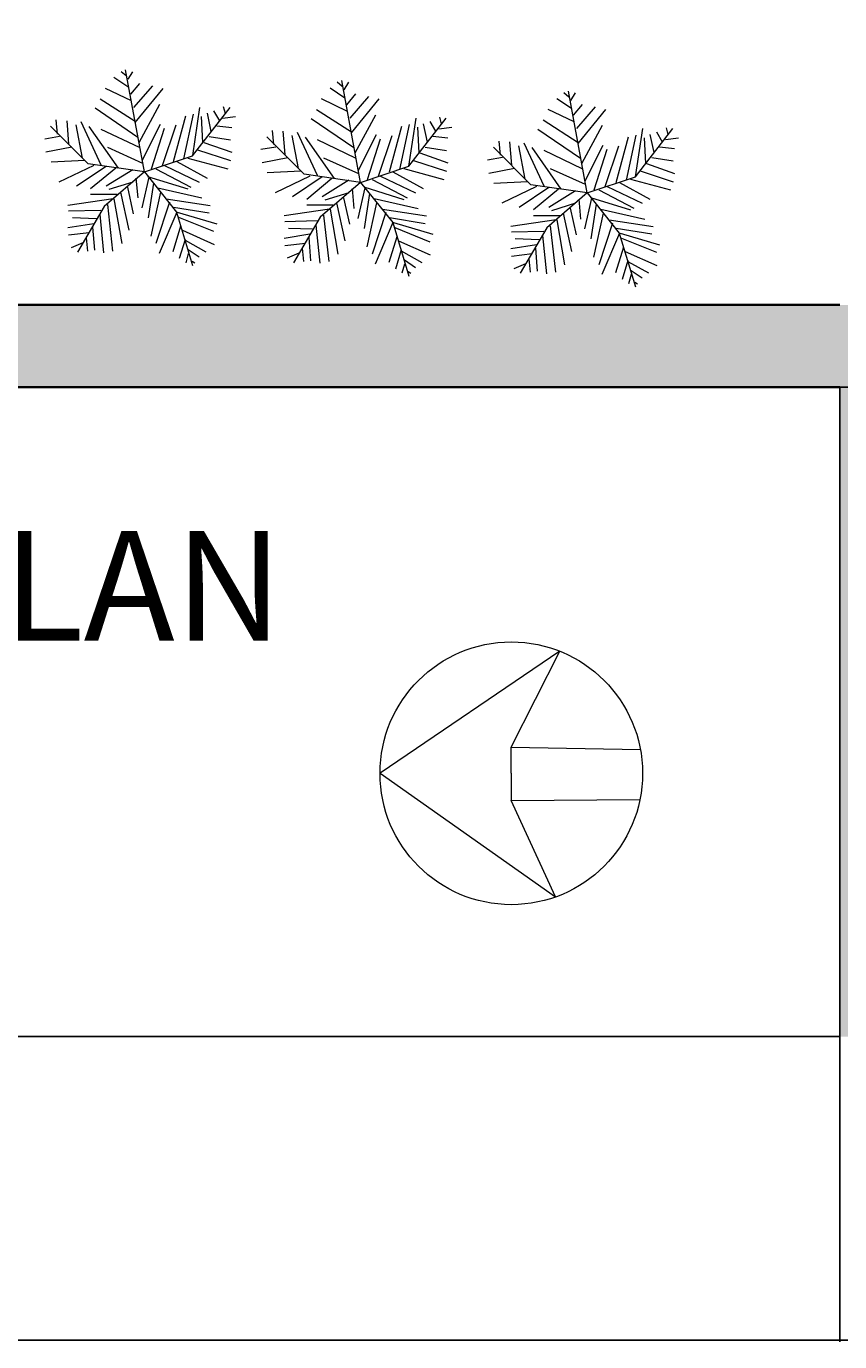
# Model space of a CAD drawing. Units: inches. Extents: x 2070 to 4408, y 1595 to 4269.
# Tile 4 of 20: x 2247 to 2336, y 1595 to 1739. Entities that reach past the tile are written whole.
import ezdxf

# ---------------------------------------------------------------- set-up
doc = ezdxf.new("R2010")
doc.units = ezdxf.units.IN
for name, color, linetype, lineweight in [('A-ANNO-DIMS', 2, 'Continuous', 18), ('A-ANNO-SYMB', 7, 'Continuous', 18), ('A-ANNO-TITL', 7, 'Continuous', 25), ('A-WALL', 7, 'Continuous', 35), ('L-PLNT', 3, 'Continuous', 13)]:
    doc.layers.add(name, color=color, linetype=linetype, lineweight=lineweight)
doc.layers.add('A-WALL-PATT', color=18, linetype='Continuous', lineweight=13, true_color=0x000000)
doc.styles.get("Standard").update_dxf_attribs({"font": 'arial.ttf'})
doc.dimstyles.get("Standard").update_dxf_attribs({"dimtxt": 0.18, "dimasz": 0.18, "dimexe": 0.18, "dimexo": 0.0625, "dimgap": 0.09, "dimtad": 0, "dimtih": 1, "dimtoh": 1, "dimdec": 4, "dimzin": 0, "dimdsep": 46, "dimtxsty": 'Standard', "dimcen": 0.09, "dimadec": 0, "dimazin": 0, "dimtfac": 1, "dimtdec": 4, "dimtofl": 0, "dimtmove": 0, "dimatfit": 3, "dimfxl": 1, "dimtolj": 1, "dimtzin": 0, "dimarcsym": 0})

# ---------------------------------------------------------------- blocks, each defined once
blk = doc.blocks.new('Trees - Imperial')
for p, q in [((-8.737, 47.138), (-17.069, 52.711)), ((-10.186, 53.64), (-13.084, 55.962)), ((0, 0), (-10.5, 57)), ((-9.099, 51.782), (-6.563, 55.962)), ((-7.288, 39.707), (-21.778, 46.673)), ((-7.65, 43.423), (-2.578, 49.46)), ((-5.839, 35.992), (4.667, 48.067)), ((-5.114, 27.632), (10.463, 46.673)), ((-5.114, 28.097), (-24.676, 40.636)), ((-2.941, 16.486), (8.652, 37.85)), ((-3.665, 19.273), (-27.574, 35.527)), ((16.259, 5.805), (23.142, 31.348)), ((22.055, 7.198), (27.489, 32.277)), ((27, 9), (48, 36)), ((27.127, 9.056), (31.112, 35.992)), ((31.836, 30.883), (32.561, 16.486)), ((35.096, 32.741), (37.27, 22.524)), ((38.719, 34.134), (41.979, 28.561)), ((43.791, 29.954), (51.036, 30.883)), ((44.153, 36.456), (45.239, 32.741)), ((-31.5, 4.5), (-52.5, 25.5)), ((-48.585, 21.131), (-49.309, 29.026)), ((-43.513, 28.561), (-42.427, 15.558)), ((-38.442, 26.239), (-34.819, 7.663)), ((-35.544, 28.097), (-24.314, 3.947)), ((-14.533, 2.09), (-30.834, 25.31)), ((-24.314, 23.917), (-2.941, 13.7)), ((-1.129, 6.734), (9.014, 26.704)), ((3.942, 1.625), (11.187, 24.381)), ((10.101, 3.483), (17.708, 26.239)), ((40.53, 25.775), (48.862, 24.846)), ((-47.498, 19.737), (-55.83, 18.344)), ((33.285, 16.486), (48.862, 10.913)), ((36.183, 19.737), (48.137, 17.88)), ((-40.615, 13.7), (-55.105, 10.913)), ((-20.691, 13.7), (-1.129, 4.876)), ((0, 0), (27, 9)), ((24.229, 7.663), (46.688, 1.625)), ((29.662, 12.307), (48.137, 6.269)), ((-33.37, 6.269), (-52.207, 5.34)), ((-28.299, 3.483), (-47.86, -5.805)), ((-21.416, 3.018), (-38.079, -8.128)), ((0, 0), (-31.5, 4.5)), ((-15.982, 2.09), (-30.11, -9.521)), ((0, 0), (-22.5, -19.5)), ((-6.563, 1.161), (-21.416, -8.128)), ((0, 0), (18, -22.5)), ((6.478, 1.625), (26.04, -8.592)), ((11.187, 3.483), (30.749, -5.805)), ((18.07, 5.805), (35.096, -3.483)), ((-6.563, -5.805), (-19.967, -9.985)), ((-4.752, -3.483), (-3.665, -14.629)), ((2.493, -3.019), (-1.491, -20.202)), ((1.769, -2.555), (24.229, -9.521)), ((5.029, -6.27), (2.131, -25.775)), ((-15.257, -12.772), (-30.11, -12.772)), ((-13.446, -11.378), (-8.737, -32.741)), ((-9.461, -8.592), (-6.201, -23.453)), ((9.014, -11.378), (3.58, -35.992)), ((7.565, -9.056), (32.198, -14.629)), ((-17.431, -15.094), (-42.789, -18.809)), ((-24.314, -21.596), (-42.427, -22.06)), ((-22.5, -19.5), (-37.5, -45)), ((-20.691, -18.345), (-17.793, -44.352)), ((-17.069, -15.094), (-12.721, -40.172)), ((14.085, -16.951), (6.478, -40.172)), ((12.274, -15.094), (36.907, -18.809)), ((16.259, -19.738), (36.183, -22.989)), ((-28.299, -29.026), (-42.789, -31.348)), ((-26.849, -26.24), (-40.253, -25.775)), ((-25.038, -23.918), (-22.865, -45.281)), ((18.07, -22.524), (8.289, -45.745)), ((18, -22.5), (27, -52.5)), ((18.433, -22.524), (40.53, -29.026)), ((19.157, -25.311), (38.719, -33.206)), ((-30.834, -34.135), (-42.427, -35.528)), ((-29.023, -30.884), (-27.936, -43.887)), ((20.244, -30.419), (15.897, -44.816)), ((21.331, -32.741), (39.081, -40.636)), ((-34.457, -39.708), (-40.978, -42.494)), ((-32.646, -36.921), (-31.921, -44.352)), ((22.78, -37.85), (19.519, -48.532)), ((22.78, -38.314), (34.372, -44.816)), ((24.591, -43.423), (30.749, -47.603)), ((24.591, -45.745), (23.142, -50.854)), ((26.764, -49.925), (28.213, -50.854))]:
    blk.add_line(p, q)
blk = doc.blocks.new('*D24')
at = {"layer": 'A-ANNO-DIMS', "color": 0, "lineweight": -2, "transparency": 16777216}
for p, q in [((2103.13, 2291.4), (2069.84, 2291.4)), ((2070.02, 2291.22), (2070.02, 1960.08)), ((2070.02, 1628.58), (2070.02, 1959.72)), ((2336.13, 1628.4), (2069.84, 1628.4))]:
    blk.add_line(p, q, dxfattribs=at)
at = {"layer": 'A-ANNO-DIMS', "color": 0, "transparency": 16777216}
for points in [[(2069.99, 2291.22), (2070.05, 2291.22), (2070.02, 2291.4)], [(2069.99, 1628.58), (2070.05, 1628.58), (2070.02, 1628.4)]]:
    blk.add_solid(points, dxfattribs=at)
at = {"layer": 'Defpoints', "color": 0, "transparency": 16777216}
for p in [(2070.02, 2291.4), (2103.2, 2291.4), (2336.2, 1628.4)]:
    blk.add_point(p, dxfattribs=at)
at = {"layer": 'A-ANNO-DIMS', "color": 0, "transparency": 16777216, "insert": (2070.02, 1959.9), "char_height": 0.18, "attachment_point": 5}
blk.add_mtext('\\A1;663', dxfattribs=at)
blk = doc.blocks.new('*D25')
at = {"layer": 'A-ANNO-DIMS', "color": 0, "lineweight": -2, "transparency": 16777216}
for p, q in [((2103.2, 1699.34), (2103.2, 1595.04)), ((2336.2, 1699.34), (2336.2, 1595.04)), ((2103.38, 1595.22), (2219.41, 1595.22)), ((2336.02, 1595.22), (2219.99, 1595.22))]:
    blk.add_line(p, q, dxfattribs=at)
at = {"layer": 'A-ANNO-DIMS', "color": 0, "transparency": 16777216}
for points in [[(2103.38, 1595.25), (2103.38, 1595.19), (2103.2, 1595.22)], [(2336.02, 1595.25), (2336.02, 1595.19), (2336.2, 1595.22)]]:
    blk.add_solid(points, dxfattribs=at)
at = {"layer": 'Defpoints', "color": 0, "transparency": 16777216}
for p in [(2103.2, 1699.4), (2336.2, 1699.4), (2336.2, 1595.22)]:
    blk.add_point(p, dxfattribs=at)
at = {"layer": 'A-ANNO-DIMS', "color": 0, "transparency": 16777216, "insert": (2219.7, 1595.22), "char_height": 0.18, "attachment_point": 5}
blk.add_mtext('\\A1;233', dxfattribs=at)
blk = doc.blocks.new('*D26')
at = {"layer": 'A-ANNO-DIMS', "color": 0, "lineweight": -2, "transparency": 16777216}
for p, q in [((2336.26, 1699.4), (2488.56, 1699.4)), ((2488.38, 1699.22), (2488.38, 1664.08)), ((2488.38, 1628.58), (2488.38, 1663.72)), ((2454.95, 1628.4), (2488.56, 1628.4))]:
    blk.add_line(p, q, dxfattribs=at)
at = {"layer": 'A-ANNO-DIMS', "color": 0, "transparency": 16777216}
for points in [[(2488.35, 1699.22), (2488.41, 1699.22), (2488.38, 1699.4)], [(2488.35, 1628.58), (2488.41, 1628.58), (2488.38, 1628.4)]]:
    blk.add_solid(points, dxfattribs=at)
at = {"layer": 'Defpoints', "color": 0, "transparency": 16777216}
for p in [(2336.2, 1699.4), (2488.38, 1699.4), (2454.88, 1628.4)]:
    blk.add_point(p, dxfattribs=at)
at = {"layer": 'A-ANNO-DIMS', "color": 0, "transparency": 16777216, "insert": (2488.38, 1663.9), "char_height": 0.18, "attachment_point": 5}
blk.add_mtext('\\A1;71', dxfattribs=at)
blk = doc.blocks.new('*D27')
at = {"layer": 'A-ANNO-DIMS', "color": 0, "lineweight": -2, "transparency": 16777216}
for p, q in [((2345.2, 1637.34), (2345.2, 1595.04)), ((2336.2, 1628.34), (2336.2, 1595.04)), ((2336.38, 1595.22), (2340.55, 1595.22)), ((2345.02, 1595.22), (2340.85, 1595.22))]:
    blk.add_line(p, q, dxfattribs=at)
at = {"layer": 'A-ANNO-DIMS', "color": 0, "transparency": 16777216}
for points in [[(2336.38, 1595.25), (2336.38, 1595.19), (2336.2, 1595.22)], [(2345.02, 1595.25), (2345.02, 1595.19), (2345.2, 1595.22)]]:
    blk.add_solid(points, dxfattribs=at)
at = {"layer": 'Defpoints', "color": 0, "transparency": 16777216}
for p in [(2345.2, 1637.4), (2336.2, 1628.4), (2345.2, 1595.22)]:
    blk.add_point(p, dxfattribs=at)
at = {"layer": 'A-ANNO-DIMS', "color": 0, "transparency": 16777216, "insert": (2340.7, 1595.22), "char_height": 0.18, "attachment_point": 5}
blk.add_mtext('\\A1;9', dxfattribs=at)
blk = doc.blocks.new('*D32')
at = {"layer": 'A-ANNO-DIMS', "color": 0, "lineweight": -2, "transparency": 16777216}
for p, q in [((2245.2, 2230.58), (2245.2, 1595.04)), ((2340.2, 2230.58), (2340.2, 1595.04)), ((2245.38, 1595.22), (2292.48, 1595.22)), ((2340.02, 1595.22), (2292.92, 1595.22))]:
    blk.add_line(p, q, dxfattribs=at)
at = {"layer": 'A-ANNO-DIMS', "color": 0, "transparency": 16777216}
for points in [[(2245.38, 1595.25), (2245.38, 1595.19), (2245.2, 1595.22)], [(2340.02, 1595.25), (2340.02, 1595.19), (2340.2, 1595.22)]]:
    blk.add_solid(points, dxfattribs=at)
at = {"layer": 'Defpoints', "color": 0, "transparency": 16777216}
for p in [(2245.2, 2230.65), (2340.2, 2230.65), (2340.2, 1595.22)]:
    blk.add_point(p, dxfattribs=at)
at = {"layer": 'A-ANNO-DIMS', "color": 0, "transparency": 16777216, "insert": (2292.7, 1595.22), "char_height": 0.18, "attachment_point": 5}
blk.add_mtext('\\A1;95', dxfattribs=at)

msp = doc.modelspace()

# ---------------------------------------------------------------- hatches: boundary and pattern name
at = {"layer": 'A-WALL-PATT'}
h = msp.add_hatch(color=256, dxfattribs=at)
h.dxf.hatch_style = 1
h.paths.add_polyline_path([(2346.196, 2218.3995), (2346.196, 2282.3995), (2340.196, 2282.3995), (2340.196, 2212.3995), (2345.5866, 2212.3995), (2346.196, 2212.3995)], flags=0)
h.paths.add_polyline_path([(2245.196, 2282.3995), (2239.196, 2282.3995), (2239.196, 2186.3995), (2244.5866, 2186.3995), (2245.196, 2186.3995)], flags=0)
h.paths.add_polyline_path([(2340.196, 2230.6455), (2245.196, 2230.6455), (2245.196, 2224.6455), (2340.196, 2224.6455)], flags=0)
h.paths.add_polyline_path([(2245.196, 2150.3995), (2239.196, 2150.3995), (2164.4362, 2150.3995), (2164.4362, 2144.3995), (2239.196, 2144.3995), (2239.196, 2086.3995), (2239.196, 2067.2711), (2244.5866, 2067.2711), (2245.196, 2067.2711), (2245.196, 2144.3995)], flags=0)
h.paths.add_polyline_path([(2346.196, 2176.3995), (2340.196, 2176.3995), (2340.196, 2086.3995), (2346.196, 2086.3995), (2346.196, 2125.318)], flags=0)
h.paths.add_polyline_path([(2446.196, 2086.3995), (2346.196, 2086.3995), (2340.196, 2086.3995), (2340.196, 2080.3995), (2446.196, 2080.3995)], flags=0)
h.paths.add_polyline_path([(2455.196, 2291.3995), (2103.196, 2291.3995), (2103.196, 1699.3995), (2336.196, 1699.3995), (2336.196, 1628.3995), (2345.196, 1628.3995), (2446.196, 1628.3995), (2454.8846, 1628.3995), (2454.8846, 1699.3995)])
h.paths.add_polyline_path([(2446.196, 2282.3995), (2446.196, 2218.3995), (2446.196, 2212.3995), (2446.196, 2086.3995), (2446.196, 2080.3995), (2446.196, 1708.3995), (2446.196, 1637.3995), (2345.196, 1637.3995), (2345.196, 1699.3995), (2345.196, 1708.3995), (2336.196, 1708.3995), (2112.196, 1708.3995), (2112.196, 2282.3995), (2239.196, 2282.3995), (2245.196, 2282.3995), (2356.196, 2282.3995)], flags=16)
h.paths.add_polyline_path([(2245.196, 2150.3995), (2245.196, 2144.3995), (2245.196, 2067.2711), (2244.5866, 2067.2711), (2239.196, 2067.2711), (2239.196, 2065.6988), (2203.2929, 2065.6988, 0.40145271), (2239.196, 2031.3337), (2244.5866, 2031.3337), (2245.196, 2031.2711), (2245.196, 1924.1525), (2239.196, 1924.1525), (2239.196, 1922.5803), (2203.2929, 1922.5803, 0.40145271), (2239.196, 1888.2151), (2244.5866, 1888.2151), (2245.196, 1888.1525), (2245.196, 1748.3995), (2339.196, 1748.4621, -0.40145271), (2303.2929, 1782.8272), (2303.2585, 1782.8272), (2303.2585, 1784.3995), (2339.196, 1784.3995), (2339.196, 1877.2067), (2291.196, 1877.2067), (2291.196, 1883.2067), (2291.196, 1946.3995), (2291.196, 1952.3995), (2291.196, 2086.3995), (2297.196, 2086.3995), (2302.196, 2086.3995), (2302.196, 2081.0259), (2303.7633, 2081.0259), (2303.7633, 2080.3995), (2338.0148, 2080.3995, 0.00437129), (2338.0203, 2081.0259), (2338.0203, 2086.3995), (2340.196, 2086.3995), (2340.196, 2176.4621), (2345.5866, 2176.4621, 0.40145271), (2381.4896, 2210.8272), (2345.5866, 2210.8272), (2345.5866, 2212.3995), (2340.196, 2212.3995), (2340.196, 2224.6455), (2245.196, 2224.6455), (2245.196, 2186.3995), (2244.5866, 2186.3995), (2239.196, 2186.3995), (2239.196, 2184.8272), (2203.2929, 2184.8272, 0.40145271), (2239.196, 2150.4621), (2244.5866, 2150.4621)], flags=0)
h.paths.add_polyline_path([(2346.196, 2282.3995), (2346.196, 2218.3995), (2377.1813, 2218.3995), (2377.1813, 2212.3995), (2346.196, 2212.3995), (2345.5866, 2212.3995), (2340.196, 2212.3995), (2340.196, 2224.6455), (2245.196, 2224.6455), (2245.196, 2230.6455), (2245.196, 2282.3995), (2292.696, 2256.5225), (2340.196, 2282.3995)], flags=0)
h.paths.add_polyline_path([(2346.196, 2086.3995), (2340.196, 2086.3995), (2340.196, 2080.3995), (2446.196, 2080.3995), (2431.196, 2016.3995), (2446.196, 1952.3995), (2412.196, 1952.3995), (2412.196, 2080.3995), (2340.196, 2080.3995), (2340.196, 2086.3995), (2340.196, 2176.3995), (2346.196, 2176.3995), (2346.196, 2125.318)], flags=0)
h.paths.add_polyline_path([(2186.508, 2270.0471, -0.03755288), (2186.9712, 2269.8581), (2186.9164, 2270.112, -0.02759121)], flags=0)
h.paths.add_polyline_path([(2183.955, 2273.7766, 1), (2188.2945, 2273.7766, 1)], flags=0)
h.paths.add_polyline_path([(2142.5261, 2274.6158, -0.03707541), (2142.5672, 2275.1696), (2142.5672, 2276.826), (2119.8759, 2276.826), (2119.8759, 2263.0962), (2140.4332, 2263.0962), (2142.5672, 2263.0962), (2142.5672, 2274.0621, -0.03707541)], flags=0)
h.paths.add_polyline_path([(2209.8974, 2263.0962), (2209.8974, 2262.2079), (2190.8042, 2262.2079), (2190.8042, 2263.0962)], flags=0)
h.paths.add_polyline_path([(2210.6382, 2276.1833), (2210.6382, 2263.9844), (2190.2185, 2263.9844), (2190.2185, 2276.1833)], flags=0)
h.paths.add_polyline_path([(2188.4362, 2273.7766, -1), (2183.8133, 2273.7766, -1)], flags=0)
h.paths.add_polyline_path([(2245.196, 2150.3995), (2245.196, 2144.3995), (2245.196, 2067.2711), (2239.196, 2067.2711), (2239.196, 2080.3995), (2172.196, 2080.3995), (2172.196, 2000.3995), (2239.196, 2000.3995), (2239.196, 1940.3995), (2159.0187, 1940.3995), (2123.0187, 1940.3995), (2112.196, 1940.3995), (2112.196, 1946.3995), (2123.0187, 1946.3995), (2123.0187, 1982.2238), (2124.586, 1982.2238), (2124.586, 1982.1895, -0.40145271), (2158.8429, 1946.3995), (2159.0187, 1946.3995), (2239.196, 1946.3995), (2239.196, 1994.3995), (2112.196, 1994.3995), (2112.196, 2000.3995), (2139.196, 2040.3995), (2112.196, 2080.3995), (2112.196, 2086.3995), (2239.196, 2086.3995), (2239.196, 2144.3995), (2209.5809, 2144.3995), (2209.5809, 2136.3995), (2203.0809, 2136.3995), (2205.0809, 2130.3996, -0.70257121), (2199.081, 2116.3995, -0.70256205), (2193.0809, 2130.3994), (2195.0809, 2136.3995), (2192.0809, 2136.3995), (2192.0809, 2134.8995), (2189.0809, 2134.8995), (2189.0809, 2135.8995), (2191.0809, 2135.8995), (2191.0809, 2136.3995), (2188.5809, 2136.3995), (2188.5809, 2144.3995), (2164.2481, 2144.3995, -0.39385849), (2130.0035, 2109.5491), (2130.0035, 2109.5147), (2128.4362, 2109.5147), (2128.4362, 2144.3995), (2112.196, 2144.3995), (2112.196, 2150.3995), (2128.4362, 2150.3995), (2128.4362, 2150.7127), (2164.4362, 2150.7127), (2164.4362, 2150.3995), (2239.196, 2150.3995)], flags=0)
h.paths.add_polyline_path([(2188.2075, 2266.8735), (2188.2075, 2211.8632, -0.41421356), (2185.4833, 2209.1391), (2146.7995, 2209.1391, -0.41421356), (2144.0754, 2211.8632), (2144.0754, 2266.8735, -0.41421356), (2146.7995, 2269.5976), (2185.4833, 2269.5976, -0.41421356)], flags=0)
h.paths.add_polyline_path([(2185.0844, 2273.7766, -1), (2187.1651, 2273.7766, -1)], flags=0)
h.paths.add_polyline_path([(2182.0486, 2259.2932), (2168.0953, 2259.2932), (2168.0953, 2260.8424), (2163.7261, 2260.8424), (2163.7261, 2259.2932), (2149.7727, 2259.2932), (2149.7727, 2266.3352), (2163.7261, 2266.3352), (2163.7261, 2261.9839), (2168.0953, 2261.9839), (2168.0953, 2266.3352), (2182.0486, 2266.3352)], flags=0)
h.paths.add_polyline_path([(2148.2585, 2250.2051), (2153.0615, 2241.8861, 0.39807048)], flags=0)
h.paths.add_polyline_path([(2162.7572, 2247.2885), (2153.1461, 2241.7396), (2148.1083, 2250.4653), (2157.7194, 2256.0142)], flags=0)
h.paths.add_polyline_path([(2162.6726, 2247.4351, -0.39286196), (2157.8415, 2255.6313), (2157.6431, 2255.6313), (2157.8696, 2255.7541)], flags=0)
h.paths.add_polyline_path([(2164.2604, 2145.339), (2164.4362, 2144.3995), (2164.4362, 2150.3995), (2164.2604, 2150.7127)], flags=0)
h.paths.add_polyline_path([(2208.5809, 2142.6495), (2208.5809, 2138.3995, -0.41421356), (2207.8309, 2137.3995), (2190.5809, 2137.3995, -0.41421356), (2189.5809, 2138.1495), (2189.5809, 2142.3995, -0.41421356), (2190.3309, 2143.3995), (2207.5809, 2143.3995, -0.41421356)], flags=0)
h.paths.add_polyline_path([(2147.957, 2229.9119), (2154.7494, 2223.1195, 0.39807048)], flags=0)
h.paths.add_polyline_path([(2162.7165, 2230.8473), (2154.8691, 2222.9998), (2147.7446, 2230.1244), (2155.592, 2237.9718)], flags=0)
h.paths.add_polyline_path([(2162.5969, 2230.9669, -0.39807048), (2155.8044, 2237.7594)], flags=0)
h.paths.add_polyline_path([(2391.8776, 2049.9192), (2408.5766, 2049.9192), (2408.5766, 2033.2202), (2408.5766, 1983.123), (2408.5766, 1966.4239), (2391.8776, 1966.4239), (2391.8776, 1983.123), (2341.7804, 1983.123), (2341.7804, 2033.2202), (2391.8776, 2033.2202)], flags=0)
h.paths.add_polyline_path([(2144.1055, 2274.6158, 1), (2148.445, 2274.6158, 1)], flags=0)
h.paths.add_polyline_path([(2148.5867, 2274.6158, -1), (2143.9638, 2274.6158, -1)], flags=0)
h.paths.add_polyline_path([(2145.2349, 2274.6158, -1), (2147.3156, 2274.6158, -1)], flags=0)
edge = h.paths.add_edge_path(flags=0)
edge.add_ellipse((2400.5951, 2040.9436), major_axis=(-4.5109, 0), ratio=0.97544784, start_angle=180, end_angle=270, ccw=False)
edge.add_ellipse((2400.5951, 2040.9436), major_axis=(-4.5109, 0), ratio=0.97544784, start_angle=90, end_angle=180, ccw=False)
edge.add_ellipse((2400.5951, 2040.9436), major_axis=(-4.5109, 0), ratio=0.97544784, start_angle=0, end_angle=90, ccw=False)
edge.add_ellipse((2400.5951, 2040.9436), major_axis=(-4.5109, 0), ratio=0.97544784, start_angle=270, end_angle=360, ccw=False)
h.paths.add_polyline_path([(2199.0809, 2117.3995, -0.73452973), (2195.0809, 2130.3995), (2203.081, 2130.3995, -0.73453329)], flags=0)
h.paths.add_polyline_path([(2141.9147, 2276.0353), (2141.9147, 2263.9844), (2120.4685, 2263.9844), (2120.4685, 2276.0353)], flags=0)
h.paths.add_polyline_path([(2138.4481, 2273.4072), (2138.4481, 2266.7226), (2133.2801, 2266.7226), (2133.2801, 2273.4072)], flags=0)
h.paths.add_polyline_path([(2137.9691, 2272.9175), (2137.9691, 2272.204), (2135.4229, 2272.204), (2135.4229, 2271.6329), (2135.3221, 2270.1051), (2135.3221, 2269.0265), (2135.4229, 2268.6811), (2135.4229, 2267.2011), (2133.7212, 2267.2011), (2133.7212, 2268.6811), (2133.7983, 2269.9587), (2133.7983, 2271.2758), (2133.7212, 2271.6329), (2133.7212, 2273.0065), (2135.717, 2273.0065), (2135.717, 2272.9175)], flags=0)
h.paths.add_polyline_path([(2137.9215, 2271.8264), (2137.9215, 2271.3786), (2137.5182, 2271.3786), (2136.9355, 2271.3786), (2136.3529, 2271.3786), (2135.7703, 2271.3786), (2135.7703, 2271.8264), (2136.1736, 2271.8264), (2136.7562, 2271.8264), (2137.3389, 2271.8264)], flags=0)
h.paths.add_polyline_path([(2137.9215, 2271.692), (2137.5182, 2271.692), (2136.9355, 2271.513), (2137.3389, 2271.513)], flags=0)
h.paths.add_polyline_path([(2136.3529, 2271.692), (2135.7703, 2271.513), (2136.1736, 2271.513), (2136.7562, 2271.692)], flags=0)
h.paths.add_polyline_path([(2137.9215, 2271.513), (2137.5182, 2271.513), (2136.7562, 2271.747), (2136.7562, 2271.692), (2137.3389, 2271.692)], flags=0)
h.paths.add_polyline_path([(2137.8207, 2270.4664), (2137.8207, 2270.0971), (2137.8207, 2269.627), (2137.8207, 2269.1569), (2137.8207, 2268.6868), (2137.3837, 2268.6868), (2136.6442, 2268.6868), (2135.9271, 2268.6868), (2135.9271, 2269.0562), (2135.9271, 2269.5263), (2135.9271, 2269.9963), (2135.9271, 2270.4664), (2136.3641, 2270.4664), (2137.0812, 2270.4664)], flags=0)
h.paths.add_polyline_path([(2137.3837, 2269.627), (2137.8207, 2269.627), (2137.8207, 2269.5263), (2137.3837, 2269.5263), (2137.3837, 2269.1569), (2137.8207, 2269.1569), (2137.3837, 2269.0562), (2137.3837, 2268.6868), (2137.0812, 2268.6868), (2137.0812, 2269.0562), (2136.6442, 2269.0562), (2136.6442, 2268.6868), (2136.3641, 2268.6868), (2136.3641, 2269.0562), (2135.9271, 2269.0562), (2135.9271, 2269.1569), (2136.3641, 2269.1569), (2136.3641, 2269.5263), (2135.9271, 2269.5263), (2135.9271, 2269.627), (2136.3641, 2269.627), (2136.3641, 2269.9963), (2135.9271, 2269.9963), (2136.3641, 2270.0971), (2136.3641, 2270.4664), (2136.6442, 2270.4664), (2136.6442, 2270.0971), (2137.0812, 2270.0971), (2137.0812, 2270.4664), (2137.3837, 2270.4664), (2137.3837, 2270.0971), (2137.8207, 2270.0971), (2137.3837, 2269.9963)], flags=0)
h.paths.add_polyline_path([(2137.5182, 2271.8264), (2137.5182, 2271.692), (2137.3389, 2271.3786), (2137.3389, 2271.513)], flags=0)
h.paths.add_polyline_path([(2137.8179, 2267.8138), (2137.8179, 2267.6879), (2137.1876, 2267.6879), (2136.4733, 2267.6879), (2135.759, 2267.6879), (2135.759, 2267.8138), (2136.3893, 2267.8138), (2137.1036, 2267.8138)], flags=0)
h.paths.add_polyline_path([(2137.0812, 2269.9963), (2137.0812, 2269.627), (2137.0812, 2269.1569), (2136.6442, 2269.1569), (2136.6442, 2269.5263), (2136.6442, 2269.9963)], flags=0)
h.paths.add_polyline_path([(2136.3529, 2271.8264), (2136.3529, 2271.692), (2136.1736, 2271.3786), (2136.1736, 2271.513)], flags=0)
h.paths.add_polyline_path([(2136.4733, 2267.8138), (2136.4733, 2267.6879), (2136.3893, 2267.6879), (2136.3893, 2267.8138)], flags=0)
h.paths.add_polyline_path([(2407.9087, 2032.5522), (2407.9087, 1983.7909), (2359.81, 1983.7909, -0.00912788), (2359.0575, 1983.7909), (2342.4483, 1983.7909), (2342.4483, 2032.5522)], flags=0)
h.paths.add_polyline_path([(2389.1838, 2023.1358), (2353.7856, 2023.1358), (2353.7856, 1985.4867, -0.09210376), (2350.2788, 1988.655), (2350.2788, 2026.6426), (2389.1838, 2026.6426)], flags=0)
h.paths.add_polyline_path([(2352.6166, 2024.3048), (2351.4477, 2024.3048), (2351.4477, 2025.4737), (2352.6166, 2025.4737)], flags=0)
h.paths.add_polyline_path([(2399.6319, 2026.7589), (2404.3661, 2026.7589, -0.41421356), (2407.0379, 2024.087), (2407.0379, 2013.4908, -0.41421356), (2404.3661, 2010.819), (2399.6319, 2010.819, -0.41421356), (2396.96, 2013.4908), (2396.96, 2024.087, -0.41421356)], flags=0)
h.paths.add_polyline_path([(2399.6319, 2026.0909), (2404.3661, 2026.0909, -0.41421356), (2406.37, 2024.087), (2406.37, 2013.4908, -0.41421356), (2404.3661, 2011.487), (2399.6319, 2011.487, -0.41421356), (2397.628, 2013.4908), (2397.628, 2024.087, -0.41421356)], flags=0)
h.paths.add_polyline_path([(2399.6319, 2002.3217), (2404.3661, 2002.3217, -0.41421356), (2407.0379, 1999.6498), (2407.0379, 1989.0536, -0.41421356), (2404.3661, 1986.3818), (2399.6319, 1986.3818, -0.41421356), (2396.96, 1989.0536), (2396.96, 1999.6498, -0.41421356)], flags=0)
h.paths.add_polyline_path([(2399.6319, 2001.6537), (2404.3661, 2001.6537, -0.41421356), (2406.37, 1999.6498), (2406.37, 1989.0536, -0.41421356), (2404.3661, 1987.0497), (2399.6319, 1987.0497, -0.41421356), (2397.628, 1989.0536), (2397.628, 1999.6498, -0.41421356)], flags=0)
edge = h.paths.add_edge_path(flags=0)
edge.add_ellipse((2400.5951, 1975.3996), major_axis=(-4.5109, 0), ratio=0.97544784, start_angle=-180, end_angle=-90, ccw=False)
edge.add_ellipse((2400.5951, 1975.3996), major_axis=(-4.5109, 0), ratio=0.97544784, start_angle=90, end_angle=180, ccw=False)
edge.add_ellipse((2400.5951, 1975.3996), major_axis=(-4.5109, 0), ratio=0.97544784, start_angle=0, end_angle=90, ccw=False)
edge.add_ellipse((2400.5951, 1975.3996), major_axis=(-4.5109, 0), ratio=0.97544784, start_angle=-90, end_angle=0, ccw=False)
h.paths.add_polyline_path([(2345.196, 1910.3995), (2366.4386, 1910.3995), (2366.4386, 1925.4555), (2392.3856, 1925.4555), (2392.3856, 1933.5025), (2400.1399, 1925.4555), (2392.3856, 1919.8795), (2392.3856, 1925.4555), (2366.4386, 1925.4555), (2366.4386, 1910.3995), (2381.196, 1910.3995), (2405.196, 1910.3995), (2405.196, 1898.3995), (2446.196, 1898.3995), (2446.196, 1886.3995), (2405.196, 1886.3995), (2405.196, 1874.3995), (2446.196, 1874.3995), (2446.196, 1862.3995), (2405.196, 1862.3995), (2405.196, 1850.3995), (2446.196, 1850.3995), (2446.196, 1838.3995), (2405.196, 1838.3995), (2405.196, 1826.3995), (2446.196, 1826.3995), (2446.196, 1814.3995), (2405.196, 1814.3995), (2405.196, 1802.3995), (2446.196, 1802.3995), (2446.196, 1798.3995), (2446.196, 1792.3995), (2405.196, 1792.3995), (2405.196, 1910.3995), (2381.196, 1910.3995), (2381.196, 1792.3995), (2345.196, 1792.3995)], flags=0)
h.paths.add_polyline_path([(2333.0944, 1863.3993, -0.41421356), (2334.7225, 1861.7712), (2334.7225, 1859.329), (2335.2653, 1859.329, -0.41421356), (2337.4361, 1857.1582), (2337.4361, 1843.862, -0.41421356), (2335.2653, 1841.6911, -0.41421356), (2337.4361, 1839.5203), (2337.4361, 1827.5808, -0.41421356), (2335.2653, 1825.41, -0.41421356), (2337.4361, 1823.2392), (2337.4361, 1808.5862, -0.41421356), (2335.2653, 1806.4153), (2334.7225, 1806.4153), (2334.7225, 1803.9732, -0.41421356), (2333.0944, 1802.3451), (2317.356, 1802.3451), (2317.0846, 1802.3451, -0.41421356), (2315.7279, 1803.7018), (2315.7279, 1803.8646), (2313.8284, 1803.8646, -0.41421356), (2311.6576, 1806.0354), (2311.6576, 1823.2015, -0.39597602), (2313.6834, 1825.3765, -0.43384798), (2311.6576, 1827.2718), (2311.6576, 1839.761, -0.41421356), (2313.5571, 1841.6604), (2313.8284, 1841.6604), (2333.8159, 1841.6604, -0.04213623), (2334.1798, 1841.6911, -0.41421356), (2332.009, 1843.862), (2332.009, 1857.1582, -0.41421356), (2334.1798, 1859.329), (2317.356, 1859.329), (2317.0846, 1859.329, -0.41421356), (2315.7279, 1860.6858), (2315.7279, 1862.0426, -0.41421356), (2317.0846, 1863.3993), (2317.356, 1863.3993)], flags=0)
h.paths.add_polyline_path([(2208.8475, 1848.9818), (2208.8475, 1840.9741, -0.41421356), (2207.0458, 1839.1724), (2206.5453, 1839.1721), (2206.5453, 1838.7218, -0.40985861), (2204.7704, 1836.9203), (2183.7501, 1836.9203, -0.41858196), (2181.9216, 1838.7218), (2181.9216, 1839.1721), (2181.421, 1839.1724, -0.41421356), (2179.6193, 1840.9741), (2179.6193, 1848.6817, -0.44064415), (2185.1126, 1854.9874), (2203.3852, 1854.9874, -0.45707961)], flags=0)
h.paths.add_polyline_path([(2204.243, 1848.4815), (2204.243, 1848.4815, 0.41725335), (2202.2204, 1850.4833), (2186.2049, 1850.4833, 0.4111805), (2184.2237, 1848.4815), (2184.2237, 1848.4815, -0.4111807), (2186.2049, 1850.4833), (2202.2204, 1850.4833, -0.41725315)], flags=0)
h.paths.add_polyline_path([(2234.7177, 1830.228), (2234.7176, 1781.6047, -0.41421356), (2233.4381, 1780.3252), (2218.6064, 1780.3252, -0.41421356), (2217.8387, 1781.0929), (2217.8387, 1783.3961, -0.41421356), (2218.6064, 1784.1639), (2218.6065, 1796.9595, -0.41421356), (2219.886, 1798.239, -0.41421356), (2218.6065, 1799.5186), (2218.6065, 1812.3142, -0.41421356), (2219.8861, 1813.5938, -0.41421356), (2218.6065, 1814.8733), (2218.6065, 1827.6689, -0.41421356), (2217.8388, 1828.4367), (2217.8388, 1830.7399, -0.41421356), (2218.6065, 1831.5076), (2233.4382, 1831.5076, -0.41421356)], flags=0)
h.paths.add_polyline_path([(2230.6344, 1827.6689, -0.41421356), (2231.4021, 1826.9012), (2231.4021, 1784.9316, -0.41421356), (2230.6343, 1784.1639), (2221.1853, 1784.1639), (2221.1853, 1827.6689)], flags=0)
h.paths.add_polyline_path([(2222.7208, 1798.239), (2221.6971, 1798.239), (2221.6971, 1813.5938), (2222.7208, 1813.5938)], flags=0)
h.paths.add_polyline_path([(2206.5453, 1773.935), (2206.5453, 1773.4848), (2206.9457, 1773.4848), (2207.0458, 1773.4845, -0.41421356), (2208.8475, 1771.6827), (2208.8475, 1763.675, -0.44222432), (2203.6505, 1757.6695), (2185.3851, 1757.6695, -0.45508402), (2179.6193, 1763.9752), (2179.6193, 1771.6827, -0.41421356), (2181.421, 1773.4845), (2181.421, 1773.4848), (2181.9216, 1773.4848), (2181.9216, 1773.935, -0.40985861), (2183.6965, 1775.7366), (2204.7167, 1775.7366, -0.41858196)], flags=0)
h.paths.add_polyline_path([(2202.2619, 1762.1736), (2186.2464, 1762.1736, -0.41725315), (2184.2237, 1764.1754), (2184.2237, 1764.1754, 0.41725335), (2186.2464, 1762.1736), (2202.2619, 1762.1736, 0.4111805), (2204.243, 1764.1754), (2204.243, 1764.1754, -0.4111807)], flags=0)
h.paths.add_polyline_path([(2313.0034, 1713.1906), (2312.997, 1713.1697), (2313.0123, 1713.1612)], flags=0)
h.paths.add_polyline_path([(2305.7314, 1721.0488), (2305.6257, 1721.1994), (2305.4853, 1721.084)], flags=0)
h.paths.add_polyline_path([(2307.5562, 1726.1427), (2307.6186, 1726.1026), (2307.5737, 1726.0477), (2308.5692, 1720.6434), (2310.5345, 1721.2985), (2310.5721, 1721.411), (2310.6958, 1721.3523), (2313.8453, 1722.4021), (2314.9351, 1723.8033), (2314.9294, 1723.9165), (2315.0028, 1723.8903), (2313.874, 1722.4389), (2313.8697, 1722.4102), (2308.5692, 1720.6434), (2308.9864, 1720.122), (2309.0665, 1720.0971), (2309.053, 1720.0387), (2310.9235, 1717.7005), (2311.4182, 1717.6259), (2311.2918, 1717.2402), (2312.0655, 1716.2731), (2312.1081, 1716.2606), (2312.0969, 1716.2339), (2308.5692, 1720.6434), (2305.2249, 1717.745), (2305.232, 1717.704), (2305.1665, 1717.6944), (2308.5692, 1720.6434)], flags=0)
h.paths.add_polyline_path([(2288.2072, 1714.3431), (2288.2008, 1714.3222), (2288.216, 1714.3137)], flags=0)
h.paths.add_polyline_path([(2280.9352, 1722.2013), (2280.8295, 1722.3519), (2280.689, 1722.2365)], flags=0)
h.paths.add_polyline_path([(2282.76, 1727.2952), (2282.8224, 1727.2551), (2282.7775, 1727.2002), (2283.773, 1721.7959), (2285.7383, 1722.451), (2285.7759, 1722.5635), (2285.8995, 1722.5048), (2289.0491, 1723.5546), (2290.1389, 1724.9558), (2290.1332, 1725.069), (2290.2065, 1725.0428), (2289.0777, 1723.5915), (2289.0735, 1723.5628), (2283.773, 1721.7959), (2284.1901, 1721.2745), (2284.2703, 1721.2496), (2284.2567, 1721.1913), (2286.1273, 1718.8531), (2286.622, 1718.7785), (2286.4956, 1718.3927), (2287.2692, 1717.4256), (2287.3119, 1717.4131), (2287.3006, 1717.3864), (2283.773, 1721.7959), (2280.4286, 1718.8975), (2280.4357, 1718.8565), (2280.3703, 1718.8469), (2283.773, 1721.7959)], flags=0)
h.paths.add_polyline_path([(2302.0672, 1721.8694), (2301.8205, 1721.8572), (2301.7578, 1722.1787), (2299.415, 1724.5215), (2299.103, 1724.4694), (2299.0662, 1724.8703)], flags=0)
h.paths.add_polyline_path([(2264.5643, 1715.4956), (2264.5579, 1715.4747), (2264.5731, 1715.4662)], flags=0)
h.paths.add_polyline_path([(2257.2923, 1723.3538), (2257.1865, 1723.5044), (2257.0461, 1723.389)], flags=0)
h.paths.add_polyline_path([(2259.117, 1728.4477), (2259.1795, 1728.4077), (2259.1345, 1728.3527), (2260.13, 1722.9484), (2262.0954, 1723.6036), (2262.133, 1723.716), (2262.2566, 1723.6573), (2265.4061, 1724.7071), (2266.4959, 1726.1083), (2266.4902, 1726.2215), (2266.5636, 1726.1953), (2265.4348, 1724.744), (2265.4305, 1724.7153), (2260.13, 1722.9484), (2260.5472, 1722.427), (2260.6273, 1722.4022), (2260.6138, 1722.3438), (2262.4843, 1720.0056), (2262.979, 1719.931), (2262.8526, 1719.5452), (2263.6263, 1718.5781), (2263.6689, 1718.5656), (2263.6577, 1718.5389), (2260.13, 1722.9484), (2256.7857, 1720.05), (2256.7928, 1720.009), (2256.7273, 1719.9994), (2260.13, 1722.9484)], flags=0)
h.paths.add_polyline_path([(2277.2709, 1723.0219), (2277.0243, 1723.0097), (2276.9616, 1723.3312), (2274.6187, 1725.6741), (2274.3067, 1725.6219), (2274.27, 1726.0228)], flags=0)
h.paths.add_polyline_path([(2253.628, 1724.1744), (2253.3814, 1724.1622), (2253.3186, 1724.4838), (2250.9758, 1726.8266), (2250.6638, 1726.7744), (2250.627, 1727.1753)], flags=0)
h.paths.add_polyline_path([(2161.9194, 1715.4956), (2161.913, 1715.4747), (2161.9282, 1715.4662)], flags=0)
h.paths.add_polyline_path([(2154.6474, 1723.3538), (2154.5416, 1723.5044), (2154.4012, 1723.389)], flags=0)
h.paths.add_polyline_path([(2162.7899, 1724.744), (2162.7856, 1724.7153), (2157.4851, 1722.9484), (2157.9023, 1722.427), (2157.9824, 1722.4022), (2157.9689, 1722.3438), (2159.8394, 1720.0056), (2160.3341, 1719.931), (2160.2078, 1719.5452), (2160.9814, 1718.5781), (2161.024, 1718.5656), (2161.0128, 1718.5389), (2157.4851, 1722.9484), (2154.1408, 1720.05), (2154.1479, 1720.009), (2154.0824, 1719.9994), (2157.4851, 1722.9484), (2156.4721, 1728.4477), (2156.5346, 1728.4077), (2156.4896, 1728.3527), (2157.4851, 1722.9484), (2159.4505, 1723.6036), (2159.4881, 1723.716), (2159.6117, 1723.6573), (2162.7612, 1724.7071), (2163.851, 1726.1083), (2163.8453, 1726.2215), (2163.9187, 1726.1953)], flags=0)
h.paths.add_polyline_path([(2150.9831, 1724.1744), (2150.7365, 1724.1622), (2150.6738, 1724.4838), (2148.3309, 1726.8266), (2148.0189, 1726.7744), (2147.9822, 1727.1753)], flags=0)
h.paths.add_polyline_path([(2132.5099, 1716.6482), (2132.5035, 1716.6272), (2132.5187, 1716.6187)], flags=0)
h.paths.add_polyline_path([(2125.2379, 1724.5064), (2125.1322, 1724.6569), (2124.9917, 1724.5415)], flags=0)
h.paths.add_polyline_path([(2133.3804, 1725.8965), (2133.3762, 1725.8678), (2128.0757, 1724.101), (2128.4928, 1723.5795), (2128.5729, 1723.5547), (2128.5594, 1723.4963), (2130.43, 1721.1581), (2130.9246, 1721.0835), (2130.7983, 1720.6977), (2131.5719, 1719.7306), (2131.6146, 1719.7181), (2131.6033, 1719.6914), (2128.0757, 1724.101), (2124.7313, 1721.2025), (2124.7384, 1721.1615), (2124.6729, 1721.1519), (2128.0757, 1724.101), (2127.0626, 1729.6002), (2127.1251, 1729.5602), (2127.0801, 1729.5052), (2128.0757, 1724.101), (2130.041, 1724.7561), (2130.0786, 1724.8685), (2130.2022, 1724.8098), (2133.3517, 1725.8597), (2134.4415, 1727.2608), (2134.4358, 1727.3741), (2134.5092, 1727.3478)], flags=0)
h.paths.add_polyline_path([(2121.5736, 1725.3269), (2121.327, 1725.3148), (2121.2643, 1725.6363), (2118.9214, 1727.9791), (2118.6094, 1727.9269), (2118.5727, 1728.3279)], flags=0)
h.paths.add_polyline_path([(2433.3904, 1646.406), (2433.384, 1646.3851), (2433.3992, 1646.3766)], flags=0)
h.paths.add_polyline_path([(2426.1184, 1654.2642), (2426.0127, 1654.4148), (2425.8722, 1654.2994)], flags=0)
h.paths.add_polyline_path([(2427.9432, 1659.3581), (2428.0056, 1659.318), (2427.9606, 1659.2631), (2428.9562, 1653.8588), (2430.9215, 1654.514), (2430.9591, 1654.6264), (2431.0827, 1654.5677), (2434.2323, 1655.6175), (2435.322, 1657.0187), (2435.3163, 1657.1319), (2435.3897, 1657.1057), (2434.2609, 1655.6544), (2434.2567, 1655.6257), (2428.9562, 1653.8588), (2429.3733, 1653.3374), (2429.4534, 1653.3126), (2429.4399, 1653.2542), (2431.3105, 1650.916), (2431.8051, 1650.8414), (2431.6788, 1650.4556), (2432.4524, 1649.4885), (2432.4951, 1649.476), (2432.4838, 1649.4493), (2428.9562, 1653.8588), (2425.6118, 1650.9604), (2425.6189, 1650.9194), (2425.5535, 1650.9098), (2428.9562, 1653.8588)], flags=0)
h.paths.add_polyline_path([(2376.63, 1645.4912), (2376.6236, 1645.4703), (2376.6388, 1645.4617)], flags=0)
h.paths.add_polyline_path([(2369.358, 1653.3494), (2369.2523, 1653.5), (2369.1118, 1653.3845)], flags=0)
h.paths.add_polyline_path([(2371.1828, 1658.4432), (2371.2452, 1658.4032), (2371.2003, 1658.3482), (2372.1958, 1652.944), (2374.1611, 1653.5991), (2374.1987, 1653.7116), (2374.3224, 1653.6528), (2377.4719, 1654.7027), (2378.5617, 1656.1038), (2378.556, 1656.2171), (2378.6293, 1656.1908), (2377.5005, 1654.7395), (2377.4963, 1654.7108), (2372.1958, 1652.944), (2372.6129, 1652.4225), (2372.6931, 1652.3977), (2372.6795, 1652.3393), (2374.5501, 1650.0011), (2375.0448, 1649.9265), (2374.9184, 1649.5407), (2375.692, 1648.5737), (2375.7347, 1648.5611), (2375.7234, 1648.5344), (2372.1958, 1652.944), (2368.8514, 1650.0456), (2368.8586, 1650.0046), (2368.7931, 1649.995), (2372.1958, 1652.944)], flags=0)
h.paths.add_polyline_path([(2404.0947, 1645.0338), (2404.0883, 1645.0128), (2404.1035, 1645.0043)], flags=0)
h.paths.add_polyline_path([(2396.8227, 1652.892), (2396.717, 1653.0425), (2396.5765, 1652.9271)], flags=0)
h.paths.add_polyline_path([(2398.6475, 1657.9858), (2398.7099, 1657.9458), (2398.665, 1657.8908), (2399.6605, 1652.4866), (2401.6258, 1653.1417), (2401.6634, 1653.2541), (2401.7871, 1653.1954), (2404.9366, 1654.2453), (2406.0264, 1655.6464), (2406.0207, 1655.7596), (2406.094, 1655.7334), (2404.9652, 1654.2821), (2404.961, 1654.2534), (2399.6605, 1652.4866), (2400.0776, 1651.9651), (2400.1578, 1651.9403), (2400.1442, 1651.8819), (2402.0148, 1649.5437), (2402.5095, 1649.4691), (2402.3831, 1649.0833), (2403.1567, 1648.1162), (2403.1994, 1648.1037), (2403.1881, 1648.077), (2399.6605, 1652.4866), (2396.3162, 1649.5881), (2396.3233, 1649.5471), (2396.2578, 1649.5375), (2399.6605, 1652.4866)], flags=0)
h.paths.add_polyline_path([(2419.4532, 1658.0857), (2422.4541, 1655.0848), (2422.2075, 1655.0726), (2422.1448, 1655.3941), (2419.8019, 1657.737), (2419.4899, 1657.6848)], flags=0)
h.paths.add_polyline_path([(2390.1575, 1656.7135), (2393.1584, 1653.7125), (2392.9118, 1653.7004), (2392.8491, 1654.0219), (2390.5063, 1656.3647), (2390.1943, 1656.3125)], flags=0)
h.paths.add_polyline_path([(2362.6928, 1657.1709), (2365.6937, 1654.1699), (2365.4471, 1654.1578), (2365.3844, 1654.4793), (2363.0416, 1656.8221), (2362.7295, 1656.77)], flags=0)
h.paths.add_polyline_path([(2419.9523, 2037.8601), (2440.2872, 2037.8601), (2440.2872, 2047.1732), (2419.9523, 2047.1732)], flags=8)
h.paths.add_polyline_path([(2370.186, 1698.9005), (2413.6287, 1698.9005), (2413.6287, 1708.0908), (2370.186, 1708.0908)], flags=8)
h.paths.add_polyline_path([(2370.1656, 1708.5185), (2430.0857, 1708.5185), (2430.0857, 1717.8316), (2370.1656, 1717.8316)], flags=8)
h.paths.add_polyline_path([(2254.1469, 1788.1883), (2302.2471, 1788.1883), (2302.2471, 1797.3786), (2254.1469, 1797.3786)], flags=8)
h.paths.add_polyline_path([(2254.1264, 1797.8063), (2326.1448, 1797.8063), (2326.1448, 1807.1194), (2254.1264, 1807.1194)], flags=8)
h.paths.add_polyline_path([(2300.08, 1914.5069), (2338.861, 1914.5069), (2338.861, 1923.6972), (2300.08, 1923.6972)], flags=8)
h.paths.add_polyline_path([(2300.0595, 1924.1249), (2331.5882, 1924.1249), (2331.5882, 1933.438), (2300.0595, 1933.438)], flags=8)
h.paths.add_polyline_path([(2176.6905, 1716.4567), (2224.1441, 1716.4567), (2224.1441, 1725.647), (2176.6905, 1725.647)], flags=8)
h.paths.add_polyline_path([(2176.67, 1726.0747), (2245.9176, 1726.0747), (2245.9176, 1735.3878), (2176.67, 1735.3878)], flags=8)
h.paths.add_polyline_path([(2339.997, 2039.7696), (2388.1034, 2039.7696), (2388.1034, 2048.9661), (2339.997, 2048.9661)], flags=8)
h.paths.add_polyline_path([(2339.9776, 2049.3928), (2388.7204, 2049.3928), (2388.7204, 2058.7059), (2339.9776, 2058.7059)], flags=8)
h.paths.add_polyline_path([(2366.0063, 2161.3825), (2409.449, 2161.3825), (2409.449, 2170.5728), (2366.0063, 2170.5728)], flags=8)
h.paths.add_polyline_path([(2365.9868, 2171.0016), (2405.879, 2171.0016), (2405.879, 2180.3085), (2365.9868, 2180.3085)], flags=8)
h.paths.add_polyline_path([(2366.0102, 2247.0726), (2407.12, 2247.0726), (2407.12, 2256.263), (2366.0102, 2256.263)], flags=8)
h.paths.add_polyline_path([(2365.9897, 2256.6906), (2397.9686, 2256.6906), (2397.9686, 2266.0037), (2365.9897, 2266.0037)], flags=8)
h.paths.add_polyline_path([(2271.8465, 2102.7885), (2307.6541, 2102.7885), (2307.6541, 2111.9849), (2271.8465, 2111.9849)], flags=8)
h.paths.add_polyline_path([(2271.8281, 2112.4126), (2304.2673, 2112.4126), (2304.2673, 2121.7196), (2271.8281, 2121.7196)], flags=8)
h.paths.add_polyline_path([(2141.6408, 2187.5934), (2182.108, 2187.5934), (2182.108, 2196.7837), (2141.6408, 2196.7837)], flags=8)
h.paths.add_polyline_path([(2141.6203, 2197.2114), (2190.3631, 2197.2114), (2190.3631, 2206.5245), (2141.6203, 2206.5245)], flags=8)
h.paths.add_polyline_path([(2165.7271, 2103.039), (2211.5027, 2103.039), (2211.5027, 2112.2293), (2165.7271, 2112.2293)], flags=8)
h.paths.add_polyline_path([(2165.7077, 2112.658), (2185.1033, 2112.658), (2185.1033, 2121.965), (2165.7077, 2121.965)], flags=8)
h.paths.add_polyline_path([(2174.945, 2048.0789), (2211.3973, 2048.0789), (2211.3973, 2057.2693), (2174.945, 2057.2693)], flags=8)
h.paths.add_polyline_path([(2174.9256, 2057.698), (2194.3212, 2057.698), (2194.3212, 2067.0049), (2174.9256, 2067.0049)], flags=8)
h.paths.add_polyline_path([(2164.8305, 1965.8394), (2202.9649, 1965.8394), (2202.9649, 1975.0297), (2164.8305, 1975.0297)], flags=8)
h.paths.add_polyline_path([(2164.8111, 1975.4584), (2184.2067, 1975.4584), (2184.2067, 1984.7654), (2164.8111, 1984.7654)], flags=8)
h.paths.add_polyline_path([(2133.0392, 1862.086), (2173.5065, 1862.086), (2173.5065, 1871.2763), (2133.0392, 1871.2763)], flags=8)
h.paths.add_polyline_path([(2133.0709, 1871.8585), (2157.0382, 1871.8585), (2157.0382, 1880.8585), (2133.0709, 1880.8585)], flags=8)
h.paths.add_polyline_path([(2406.4423, 1923.5541), (2418.8209, 1923.5541), (2418.8209, 1932.7199), (2406.4423, 1932.7199)], flags=8)

# ---------------------------------------------------------------- linework, layer by layer
at = {"layer": 'A-ANNO-SYMB'}
for p, q in [((2305.5858, 1670.527), (2285.9052, 1657.1843)), ((2300.2684, 1660.0403), (2305.5858, 1670.527)), ((2300.2684, 1657.1843), (2300.2684, 1660.0403)), ((2300.2684, 1660.0403), (2314.3932, 1659.7905)), ((2285.9052, 1657.1843), (2305.1074, 1643.6608)), ((2300.2684, 1657.1843), (2300.2684, 1654.2205)), ((2300.2684, 1654.2205), (2314.344, 1654.3244)), ((2305.1074, 1643.6608), (2300.2684, 1654.2205))]:
    msp.add_line(p, q, dxfattribs=at)
msp.add_circle((2300.2684, 1657.1843), 14.3632, dxfattribs=at)
at = {"layer": 'A-WALL'}
for points in [[(2336.196, 1699.3995), (2103.196, 1699.3995), (2103.196, 2291.3995), (2455.196, 2291.3995), (2455.196, 1699.3995), (2454.8846, 1699.3995)], [(2336.196, 1708.3995), (2112.196, 1708.3995), (2112.196, 2282.3995), (2446.196, 2282.3995), (2446.196, 2218.3995)]]:
    msp.add_lwpolyline(points, dxfattribs=at)

# ---------------------------------------------------------------- block references
at = {"layer": 'L-PLNT', "xscale": 0.1954109391421404, "yscale": 0.1954109391421404, "zscale": 0.1954109391421404}
for p in [(2260.13, 1722.9484), (2283.773, 1721.7959), (2308.5692, 1720.6434)]:
    msp.add_blockref('Trees - Imperial', p, dxfattribs=at)

# ---------------------------------------------------------------- texts
at = {"layer": 'A-ANNO-TITL'}
msp.add_text('FIRST FLOOR PLAN', height=12, dxfattribs=at).set_placement((2130.495, 1671.6896))

# ---------------------------------------------------------------- dimensions: what is measured, and where the dimension line sits
at = {"layer": 'A-ANNO-DIMS'}
for base, p1, p2, picture, middle in [((2070.016, 2291.3995), (2336.196, 1628.3995), (2103.196, 2291.3995), '*D24', (2070.016, 1959.8995)), ((2488.376, 1699.3995), (2454.8846, 1628.3995), (2336.196, 1699.3995), '*D26', (2488.376, 1663.8995))]:
    dim = msp.add_linear_dim(base=base, p1=p1, p2=p2, angle=90, dimstyle='Standard', override={"dimdec": 0, "dimlfac": 1, "dimrnd": 0, "dimzin": 0, "dimdsep": 46, "dimlunit": 2}, dxfattribs=at)
    dim.commit()
    dim.dimension.update_dxf_attribs({"geometry": picture, "text_midpoint": middle})
for base, p1, p2, picture, middle in [((2340.196, 1595.2195), (2245.196, 2230.6455), (2340.196, 2230.6455), '*D32', (2292.696, 1595.2195)), ((2336.196, 1595.2195), (2103.196, 1699.3995), (2336.196, 1699.3995), '*D25', (2219.696, 1595.2195)), ((2345.196, 1595.2195), (2336.196, 1628.3995), (2345.196, 1637.3995), '*D27', (2340.696, 1595.2195))]:
    dim = msp.add_linear_dim(base=base, p1=p1, p2=p2, dimstyle='Standard', override={"dimdec": 0, "dimlfac": 1, "dimrnd": 0, "dimzin": 0, "dimdsep": 46, "dimlunit": 2}, dxfattribs=at)
    dim.commit()
    dim.dimension.update_dxf_attribs({"geometry": picture, "text_midpoint": middle})

doc.saveas('drawing.dxf')
